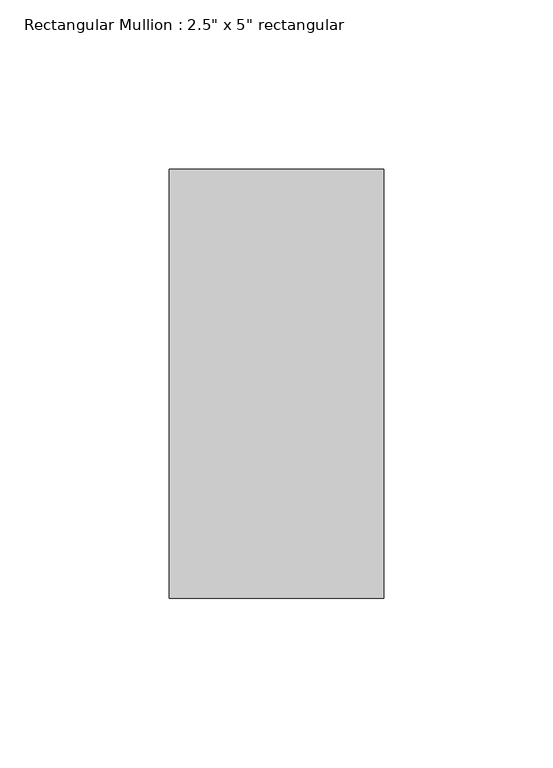
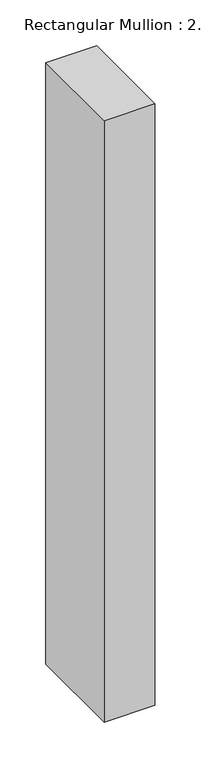
"""IFC4 building model written with IfcOpenShell, lengths in millimetres: member geometry."""

from ifc_helpers import new_model, si_unit, frame, origin, place, context, project, spatial, polyline, outline, extrude, source, transform, mapped, element, save


def member_f274020e(model_context):
    return source(origin(), model_context, "Body", "SweptSolid", [
        extrude(outline(polyline([(0.0, 63.5), (0.0, -63.5), (-63.5, -63.5), (-63.5, 63.5), (0.0, 63.5)])), frame((0.0, 0.0, -798.5443895), z_axis=(0.0, 0.0, 1.0), x_axis=(1.0, 0.0, 0.0)), (0.0, 0.0, 1.0), 798.5443895),
    ])


if __name__ == "__main__":
    model = new_model("IFC4")
    model_context = context("Model", 3, world=origin())
    ifc_project = project(units=[si_unit("LENGTHUNIT", "METRE", prefix="MILLI")], contexts=[model_context])
    site = spatial("IfcSite", under=ifc_project)
    building = spatial("IfcBuilding", under=site)
    placement = place(None, origin())
    member_shape = member_f274020e(model_context)
    element("IfcMember", 1, ObjectType="Rectangular Mullion : 2.5\" x 5\" rectangular", at=placement, inside=building, context=model_context, shape_type="MappedRepresentation", body=[
        mapped(member_shape, transform((0.0, 0.0, 0.0), x_axis=(1.0, 0.0, 0.0), y_axis=(0.0, 1.0, 0.0), z_axis=(0.0, 0.0, 1.0))),
    ])
    save(model, "model.ifc")

# Revit data of these elements
# Type "Rectangular Mullion : 2.5\" x 5\" rectangular"
#   built-in parameter 1007304 = 0.416667 (stored number, unit not read)
#   built-in parameter 1007301 = 0.104167 (stored number, unit not read)
#   built-in parameter 1007300 = 0.104167 (stored number, unit not read)
# Element 1 (IfcMember, "Rectangular Mullion : 2.5\" x 5\" rectangular")
#   Materials on its faces: "Aluminum"
# Materials
#   "Aluminum": class "Metal", colour RGB 247 247 247, transparency 0, Description = "Aluminum 6061", Cost = 0
